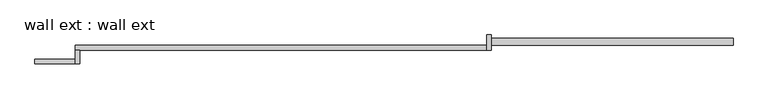
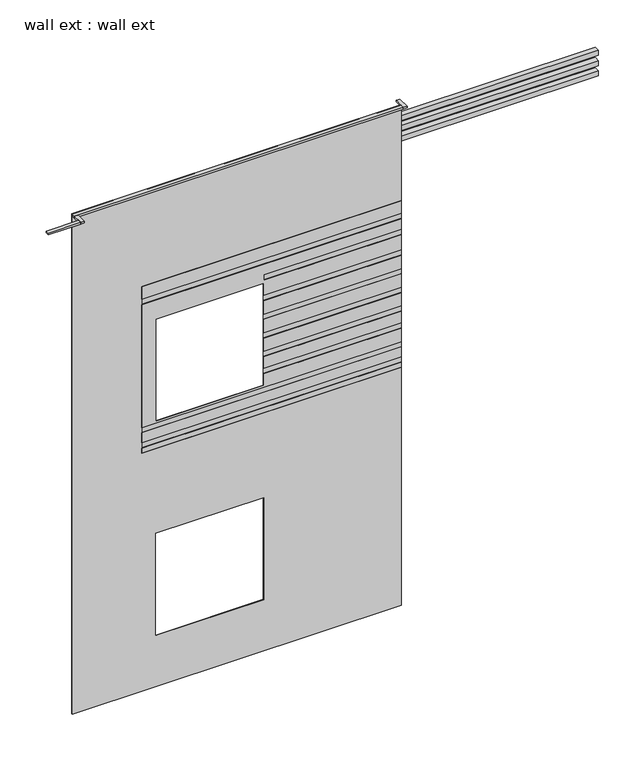
"""IFC4 building model written with IfcOpenShell, lengths in millimetres: proxy geometry, wall ext : wall ext."""

from ifc_helpers import new_model, si_unit, frame, origin, place, context, project, spatial, polyline, outline, extrude, faceted_brep, source, transform, mapped, element, save


def wall_ext_wall_ext_517f0dc9(model_context):
    return source(origin(), model_context, "Body", "SolidModel", [
        extrude(outline(polyline([(-8398.1551496, -1771.697359), (-8398.1551496, -1946.9176715), (-8448.9551496, -1946.9176715), (-8448.9551496, -1771.697359), (-8398.1551496, -1771.697359)])), frame((0.0, 0.0, 7289.8), z_axis=(0.0, 0.0, 1.0), x_axis=(1.0, 0.0, 0.0)), (0.0, 0.0, 1.0), 25.4),
        extrude(outline(polyline([(-5661.3051496, -1809.797359), (-5661.3051496, -1885.997359), (-8448.9551496, -1885.997359), (-8448.9551496, -1809.797359), (-5661.3051496, -1809.797359)])), frame((0.0, 0.0, 7077.8469628), z_axis=(0.0, 0.0, 1.0), x_axis=(1.0, 0.0, 0.0)), (0.0, 0.0, 1.0), 76.2),
        extrude(outline(polyline([(-5661.3051496, -1809.797359), (-5661.3051496, -1885.997359), (-8448.9551496, -1885.997359), (-8448.9551496, -1809.797359), (-5661.3051496, -1809.797359)])), frame((0.0, 0.0, 6925.4469628), z_axis=(0.0, 0.0, 1.0), x_axis=(1.0, 0.0, 0.0)), (0.0, 0.0, 1.0), 76.2),
        extrude(outline(polyline([(-5661.3051496, -1809.797359), (-5661.3051496, -1885.997359), (-8448.9551496, -1885.997359), (-8448.9551496, -1809.797359), (-5661.3051496, -1809.797359)])), frame((0.0, 0.0, 6773.0469628), z_axis=(0.0, 0.0, 1.0), x_axis=(1.0, 0.0, 0.0)), (0.0, 0.0, 1.0), 76.2),
        extrude(outline(polyline([(-13046.3551496, -1946.9176715), (-13046.3551496, -2098.4916291), (-13097.1551496, -2098.4916291), (-13097.1551496, -1946.9176715), (-13046.3551496, -1946.9176715)])), frame((0.0, 0.0, 7289.8), z_axis=(0.0, 0.0, 1.0), x_axis=(1.0, 0.0, 0.0)), (0.0, 0.0, 1.0), 25.4),
        extrude(outline(polyline([(-13097.1551496, -2098.4916291), (-13554.3551496, -2098.4916291), (-13554.3551496, -2047.6916291), (-13097.1551496, -2047.6916291), (-13097.1551496, -2098.4916291)])), frame((0.0, 0.0, 7289.8), z_axis=(0.0, 0.0, 1.0), x_axis=(1.0, 0.0, 0.0)), (0.0, 0.0, 1.0), 25.4),
        extrude(outline(polyline([(-8448.9551496, -1946.9176715), (-13097.1551496, -1946.9176715), (-13097.1551496, -1885.997359), (-8448.9551496, -1885.997359), (-8448.9551496, -1946.9176715)])), frame((0.0, 0.0, 7289.8), z_axis=(0.0, 0.0, 1.0), x_axis=(1.0, 0.0, 0.0)), (0.0, 0.0, 1.0), 25.4),
        faceted_brep([(-8448.9551496, -1896.1176715, 5892.8), (-12119.3495996, -1896.1176715, 5892.8), (-12119.3495996, -1896.1176715, 5702.3), (-8448.9551496, -1896.1176715, 5702.3), (-12119.3495996, -1896.1176715, 3403.6), (-8448.9551496, -1896.1176715, 3403.6), (-8448.9551496, -1896.1176715, 3476.8126712), (-12119.3495996, -1896.1176715, 3476.8126712), (-10392.0551496, -1896.1176715, 3810.0), (-11916.0551496, -1896.1176715, 3810.0), (-11916.0551496, -1896.1176715, 5334.0), (-10392.0551496, -1896.1176715, 5334.0), (-10392.0551496, -1896.1176715, 5156.2), (-8448.9551496, -1896.1176715, 5156.2), (-8448.9551496, -1896.1176715, 5381.8126712), (-10392.0551496, -1896.1176715, 5381.8126712), (-10392.0551496, -1896.1176715, 5461.0), (-8448.9551496, -1896.1176715, 5461.0), (-8448.9551496, -1896.1176715, 5623.1126712), (-12119.3495996, -1896.1176715, 5623.1126712), (-12119.3495996, -1896.1176715, 3784.6), (-8448.9551496, -1896.1176715, 3784.6), (-8448.9551496, -1896.1176715, 3984.8126712), (-10392.0551496, -1896.1176715, 3984.8126712), (-8448.9551496, -1896.1176715, 5077.0126712), (-10392.0551496, -1896.1176715, 5077.0126712), (-10392.0551496, -1896.1176715, 4876.8), (-8448.9551496, -1896.1176715, 4876.8), (-12119.3495996, -1896.1176715, 3556.0), (-8448.9551496, -1896.1176715, 3556.0), (-8448.9551496, -1896.1176715, 3705.4126712), (-12119.3495996, -1896.1176715, 3705.4126712), (-10392.0551496, -1896.1176715, 4064.0), (-8448.9551496, -1896.1176715, 4064.0), (-8448.9551496, -1896.1176715, 4238.8126712), (-10392.0551496, -1896.1176715, 4238.8126712), (-10392.0551496, -1896.1176715, 4318.0), (-8448.9551496, -1896.1176715, 4318.0), (-8448.9551496, -1896.1176715, 4518.2126712), (-10392.0551496, -1896.1176715, 4518.2126712), (-10392.0551496, -1896.1176715, 4597.4), (-8448.9551496, -1896.1176715, 4597.4), (-8448.9551496, -1896.1176715, 4797.6126712), (-10392.0551496, -1896.1176715, 4797.6126712), (-8448.9551496, -1885.997359, 5892.8), (-8448.9551496, -1885.997359, 3403.6), (-12119.3495996, -1885.997359, 3403.6), (-12119.3495996, -1885.997359, 5892.8), (-10392.0551496, -1885.997359, 3810.0), (-10392.0551496, -1885.997359, 5334.0), (-11916.0551496, -1885.997359, 5334.0), (-11916.0551496, -1885.997359, 3810.0), (-12119.3495996, -1888.4778277, 3476.8126712), (-12119.3495996, -1888.4778277, 3556.0), (-12119.3495996, -1888.4778277, 3705.4126712), (-12119.3495996, -1888.4778277, 3784.6), (-12119.3495996, -1888.4778277, 5623.1126712), (-12119.3495996, -1888.4778277, 5702.3), (-8448.9551496, -1888.4778277, 5702.3), (-8448.9551496, -1888.4778277, 5623.1126712), (-8448.9551496, -1888.4778277, 5461.0), (-8448.9551496, -1888.4778277, 5381.8126712), (-8448.9551496, -1888.4778277, 5156.2), (-8448.9551496, -1888.4778277, 5077.0126712), (-8448.9551496, -1888.4778277, 4876.8), (-8448.9551496, -1888.4778277, 4797.6126712), (-8448.9551496, -1888.4778277, 4597.4), (-8448.9551496, -1888.4778277, 4518.2126712), (-8448.9551496, -1888.4778277, 4318.0), (-8448.9551496, -1888.4778277, 4238.8126712), (-8448.9551496, -1888.4778277, 4064.0), (-8448.9551496, -1888.4778277, 3984.8126712), (-8448.9551496, -1888.4778277, 3784.6), (-8448.9551496, -1888.4778277, 3705.4126712), (-8448.9551496, -1888.4778277, 3556.0), (-8448.9551496, -1888.4778277, 3476.8126712), (-10392.0551496, -1888.4778277, 3984.8126712), (-10392.0551496, -1888.4778277, 4064.0), (-10392.0551496, -1888.4778277, 4238.8126712), (-10392.0551496, -1888.4778277, 4318.0), (-10392.0551496, -1888.4778277, 4518.2126712), (-10392.0551496, -1888.4778277, 4597.4), (-10392.0551496, -1888.4778277, 4797.6126712), (-10392.0551496, -1888.4778277, 4876.8), (-10392.0551496, -1888.4778277, 5077.0126712), (-10392.0551496, -1888.4778277, 5156.2), (-10392.0551496, -1888.4778277, 5461.0), (-10392.0551496, -1888.4778277, 5381.8126712)], [[[0, 1, 2, 3]], [[4, 5, 6, 7]], [[8, 9, 10, 11, 12, 13, 14, 15, 16, 17, 18, 19, 20, 21, 22, 23]], [[24, 25, 26, 27]], [[28, 29, 30, 31]], [[32, 33, 34, 35]], [[36, 37, 38, 39]], [[40, 41, 42, 43]], [[44, 45, 46, 47], [48, 49, 50, 51]], [[1, 0, 44, 47]], [[47, 46, 4, 7, 52, 53, 28, 31, 54, 55, 20, 19, 56, 57, 2, 1]], [[5, 4, 46, 45]], [[45, 44, 0, 3, 58, 59, 18, 17, 60, 61, 14, 13, 62, 63, 24, 27, 64, 65, 42, 41, 66, 67, 38, 37, 68, 69, 34, 33, 70, 71, 22, 21, 72, 73, 30, 29, 74, 75, 6, 5]], [[11, 49, 48, 8, 23, 76, 77, 32, 35, 78, 79, 36, 39, 80, 81, 40, 43, 82, 83, 26, 25, 84, 85, 12]], [[8, 48, 51, 9]], [[9, 51, 50, 10]], [[49, 11, 10, 50]], [[62, 85, 84, 63]], [[63, 84, 25, 24]], [[85, 62, 13, 12]], [[74, 53, 52, 75]], [[75, 52, 7, 6]], [[53, 74, 29, 28]], [[72, 55, 54, 73]], [[73, 54, 31, 30]], [[55, 72, 21, 20]], [[70, 77, 76, 71]], [[71, 76, 23, 22]], [[77, 70, 33, 32]], [[68, 79, 78, 69]], [[69, 78, 35, 34]], [[79, 68, 37, 36]], [[66, 81, 80, 67]], [[67, 80, 39, 38]], [[81, 66, 41, 40]], [[64, 83, 82, 65]], [[65, 82, 43, 42]], [[83, 64, 27, 26]], [[60, 86, 87, 61]], [[61, 87, 15, 14]], [[87, 86, 16, 15]], [[86, 60, 17, 16]], [[58, 57, 56, 59]], [[59, 56, 19, 18]], [[57, 58, 3, 2]]]),
        faceted_brep([(-8448.9551496, -1896.1176715, 7315.2), (-13097.1551496, -1896.1176715, 7315.2), (-13097.1551496, -1896.1176715, -152.4), (-8448.9551496, -1896.1176715, -152.4), (-8448.9551496, -1896.1176715, 3403.6), (-12119.3495996, -1896.1176715, 3403.6), (-12119.3495996, -1896.1176715, 3476.8126712), (-12119.3495996, -1896.1176715, 3556.0), (-12119.3495996, -1896.1176715, 3705.4126712), (-12119.3495996, -1896.1176715, 3784.6), (-12119.3495996, -1896.1176715, 5623.1126712), (-12119.3495996, -1896.1176715, 5702.3), (-12119.3495996, -1896.1176715, 5892.8), (-8448.9551496, -1896.1176715, 5892.8), (-10392.0551496, -1896.1176715, 2133.6), (-10392.0551496, -1896.1176715, 609.6), (-11916.0551496, -1896.1176715, 609.6), (-11916.0551496, -1896.1176715, 2133.6), (-8448.9551496, -1885.997359, -152.4), (-13097.1551496, -1885.997359, -152.4), (-13097.1551496, -1885.997359, 7315.2), (-8448.9551496, -1885.997359, 7315.2), (-8448.9551496, -1885.997359, 5892.8), (-12119.3495996, -1885.997359, 5892.8), (-12119.3495996, -1885.997359, 3403.6), (-8448.9551496, -1885.997359, 3403.6), (-10392.0551496, -1885.997359, 609.6), (-10392.0551496, -1885.997359, 2133.6), (-11916.0551496, -1885.997359, 2133.6), (-11916.0551496, -1885.997359, 609.6)], [[[0, 1, 2, 3, 4, 5, 6, 7, 8, 9, 10, 11, 12, 13], [14, 15, 16, 17]], [[18, 19, 20, 21, 22, 23, 24, 25], [26, 27, 28, 29]], [[1, 0, 21, 20]], [[2, 1, 20, 19]], [[3, 2, 19, 18]], [[21, 0, 13, 22]], [[3, 18, 25, 4]], [[14, 27, 26, 15]], [[15, 26, 29, 16]], [[16, 29, 28, 17]], [[27, 14, 17, 28]], [[5, 24, 23, 12, 11, 10, 9, 8, 7, 6]], [[12, 23, 22, 13]], [[24, 5, 4, 25]]]),
    ])


if __name__ == "__main__":
    model = new_model("IFC4")
    model_context = context("Model", 3, world=origin())
    ifc_project = project(units=[si_unit("LENGTHUNIT", "METRE", prefix="MILLI")], contexts=[model_context])
    site = spatial("IfcSite", under=ifc_project)
    building = spatial("IfcBuilding", under=site)
    placement = place(None, origin())
    wall_ext_wall_ext_shape = wall_ext_wall_ext_517f0dc9(model_context)
    element("IfcBuildingElementProxy", 1, Name="wall ext : wall ext", ObjectType="wall ext : wall ext", at=placement, inside=building, context=model_context, shape_type="MappedRepresentation", body=[
        mapped(wall_ext_wall_ext_shape, transform((0.0, 0.0, 0.0), x_axis=(1.0, 0.0, 0.0), y_axis=(0.0, 1.0, 0.0), z_axis=(0.0, 0.0, 1.0))),
    ])
    save(model, "model.ifc")

# Revit data of these elements
# Element 1 (IfcBuildingElementProxy, "wall ext : wall ext")
#   Materials on its faces: "Door - Frame", "Damp-proofing", "wall"
# Materials
#   "Door - Frame": colour RGB 118 70 51, transparency 0, Cost = 0
#   "Damp-proofing": class "Generic", colour RGB 127 127 127, transparency 0, Description = "Damp-proofing", Cost = 0
#   "wall": class "Generic", colour RGB 120 120 120, transparency 0, Cost = 0
